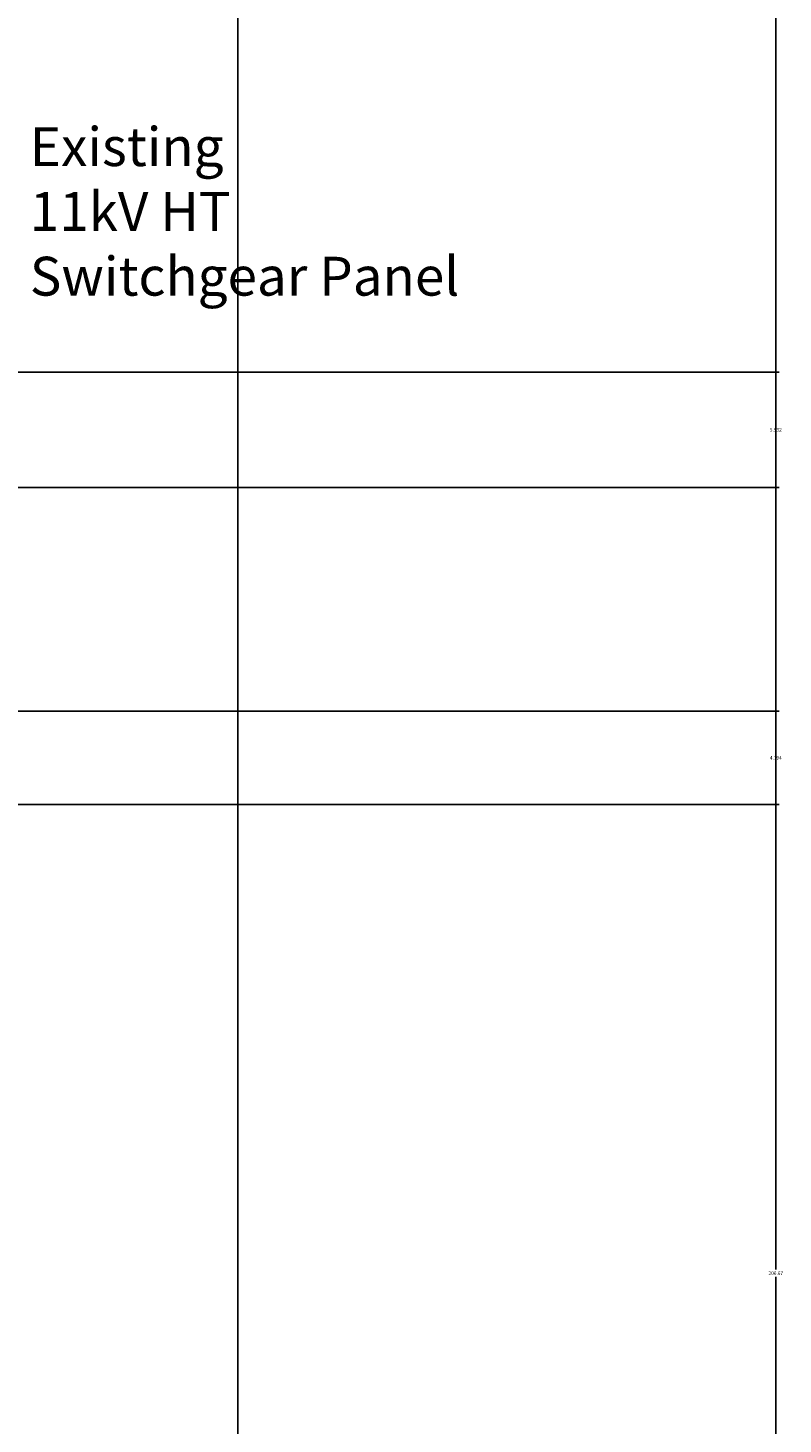
# Model space of a CAD drawing. Units: inches. Extents: x 412 to 584, y 208 to 437.
# Tile 22 of 28: x 545 to 584, y 315 to 387. Entities that reach past the tile are written whole.
import ezdxf

# ---------------------------------------------------------------- set-up
doc = ezdxf.new("R2010")
doc.units = ezdxf.units.IN
doc.header["$MEASUREMENT"] = 0
doc.layers.add('A-ANNO-DIMS', color=2, linetype='Continuous', lineweight=18)
doc.layers.add('E-ANNO-TEXT', color=7, linetype='Continuous', lineweight=18)
doc.styles.get("Standard").update_dxf_attribs({"font": 'arial.ttf'})
doc.dimstyles.get("Standard").update_dxf_attribs({"dimtxt": 0.18, "dimasz": 0.18, "dimexe": 0.18, "dimexo": 0.0625, "dimgap": 0.09, "dimtad": 0, "dimtih": 1, "dimtoh": 1, "dimdec": 4, "dimzin": 0, "dimdsep": 46, "dimtxsty": 'Standard', "dimcen": 0.09, "dimadec": 0, "dimazin": 0, "dimtfac": 1, "dimtdec": 4, "dimtofl": 0, "dimtmove": 0, "dimatfit": 3, "dimfxl": 1, "dimtolj": 1, "dimtzin": 0, "dimarcsym": 0})

# ---------------------------------------------------------------- blocks, each defined once
blk = doc.blocks.new('*D17')
at = {"layer": 'A-ANNO-DIMS', "color": 0, "lineweight": -2, "transparency": 16777216}
for p, q in [((497.715, 426.185), (583.674, 426.185)), ((583.494, 426.005), (583.494, 323.031)), ((583.494, 219.693), (583.494, 322.667)), ((550.198, 219.513), (583.674, 219.513))]:
    blk.add_line(p, q, dxfattribs=at)
at = {"layer": 'A-ANNO-DIMS', "color": 0, "transparency": 16777216}
for points in [[(583.464, 426.005), (583.524, 426.005), (583.494, 426.185)], [(583.464, 219.693), (583.524, 219.693), (583.494, 219.513)]]:
    blk.add_solid(points, dxfattribs=at)
at = {"layer": 'Defpoints', "color": 0, "transparency": 16777216}
for p in [(497.652, 426.185), (550.135, 219.513), (583.494, 219.513)]:
    blk.add_point(p, dxfattribs=at)
at = {"layer": 'A-ANNO-DIMS', "color": 0, "transparency": 16777216, "insert": (583.494, 322.849), "char_height": 0.18, "attachment_point": 5}
blk.add_mtext('\\A1;206.67', dxfattribs=at)
blk = doc.blocks.new('*D28')
at = {"layer": 'A-ANNO-DIMS', "color": 0, "lineweight": -2, "transparency": 16777216}
for p, q in [((450.562, 256.635), (450.562, 437.465)), ((450.742, 437.285), (502.724, 437.285)), ((555.616, 437.285), (503.634, 437.285)), ((555.796, 256.635), (555.796, 437.465))]:
    blk.add_line(p, q, dxfattribs=at)
at = {"layer": 'A-ANNO-DIMS', "color": 0, "transparency": 16777216}
for points in [[(450.742, 437.315), (450.742, 437.255), (450.562, 437.285)], [(555.616, 437.315), (555.616, 437.255), (555.796, 437.285)]]:
    blk.add_solid(points, dxfattribs=at)
at = {"layer": 'Defpoints', "color": 0, "transparency": 16777216}
for p in [(555.796, 437.285), (450.562, 256.573), (555.796, 256.573)]:
    blk.add_point(p, dxfattribs=at)
at = {"layer": 'A-ANNO-DIMS', "color": 0, "transparency": 16777216, "insert": (503.179, 437.285), "char_height": 0.18, "attachment_point": 5}
blk.add_mtext('\\A1;105.23', dxfattribs=at)
blk = doc.blocks.new('*D35')
at = {"layer": 'A-ANNO-DIMS', "color": 0, "lineweight": -2, "transparency": 16777216}
for p, q in [((485.523, 369.221), (583.674, 369.221)), ((583.494, 369.041), (583.494, 366.437)), ((583.494, 363.469), (583.494, 366.073)), ((485.523, 363.289), (583.674, 363.289))]:
    blk.add_line(p, q, dxfattribs=at)
at = {"layer": 'A-ANNO-DIMS', "color": 0, "transparency": 16777216}
for points in [[(583.464, 369.041), (583.524, 369.041), (583.494, 369.221)], [(583.464, 363.469), (583.524, 363.469), (583.494, 363.289)]]:
    blk.add_solid(points, dxfattribs=at)
at = {"layer": 'Defpoints', "color": 0, "transparency": 16777216}
for p in [(485.46, 369.221), (485.46, 363.289), (583.494, 363.289)]:
    blk.add_point(p, dxfattribs=at)
at = {"layer": 'A-ANNO-DIMS', "color": 0, "transparency": 16777216, "insert": (583.494, 366.255), "char_height": 0.18, "attachment_point": 5}
blk.add_mtext('\\A1;5.932', dxfattribs=at)
blk = doc.blocks.new('*D40')
at = {"layer": 'A-ANNO-DIMS', "color": 0, "lineweight": -2, "transparency": 16777216}
for p, q in [((501.747, 351.77), (583.674, 351.77)), ((583.494, 351.59), (583.494, 349.555)), ((583.494, 347.157), (583.494, 349.191)), ((501.747, 346.977), (583.674, 346.977))]:
    blk.add_line(p, q, dxfattribs=at)
at = {"layer": 'A-ANNO-DIMS', "color": 0, "transparency": 16777216}
for points in [[(583.464, 351.59), (583.524, 351.59), (583.494, 351.77)], [(583.464, 347.157), (583.524, 347.157), (583.494, 346.977)]]:
    blk.add_solid(points, dxfattribs=at)
at = {"layer": 'Defpoints', "color": 0, "transparency": 16777216}
for p in [(501.685, 351.77), (501.685, 346.977), (583.494, 346.977)]:
    blk.add_point(p, dxfattribs=at)
at = {"layer": 'A-ANNO-DIMS', "color": 0, "transparency": 16777216, "insert": (583.494, 349.373), "char_height": 0.18, "attachment_point": 5}
blk.add_mtext('\\A1;4.794', dxfattribs=at)

msp = doc.modelspace()

# ---------------------------------------------------------------- texts
at = {"layer": 'E-ANNO-TEXT', "insert": (545.0898, 381.8285), "char_height": 2, "attachment_point": 1}
msp.add_mtext_dynamic_manual_height_columns('\\pxql;Existing\\P11kV HT\\PSwitchgear Panel', width=26.749239, gutter_width=1, heights=[11.4418], dxfattribs=at)

# ---------------------------------------------------------------- dimensions: what is measured, and where the dimension line sits
at = {"layer": 'A-ANNO-DIMS'}
dim = msp.add_linear_dim(base=(555.7959, 437.2847), p1=(450.562, 256.5729), p2=(555.7959, 256.5729), dimstyle='Standard', override={"dimdec": 2, "dimlfac": 1, "dimrnd": 0, "dimzin": 0, "dimdsep": 46, "dimlunit": 2}, dxfattribs=at)
dim.commit()
dim.dimension.update_dxf_attribs({"geometry": '*D28', "text_midpoint": (503.1789, 437.2847)})
for base, p1, p2, override, picture, middle in [((583.4937, 219.5133), (497.6523, 426.1847), (550.1351, 219.5133), {"dimdec": 2, "dimlfac": 1, "dimrnd": 0, "dimzin": 0, "dimdsep": 46, "dimlunit": 2}, '*D17', (583.4937, 322.849)), ((583.4937, 363.2888), (485.4605, 369.221), (485.4605, 363.2888), {"dimdec": 3, "dimlfac": 1, "dimrnd": 0, "dimzin": 0, "dimdsep": 46, "dimlunit": 2}, '*D35', (583.4937, 366.2549)), ((583.4937, 346.9765), (501.6846, 351.7702), (501.6846, 346.9765), {"dimdec": 3, "dimlfac": 1, "dimrnd": 0, "dimzin": 0, "dimdsep": 46, "dimlunit": 2}, '*D40', (583.4937, 349.3734))]:
    dim = msp.add_linear_dim(base=base, p1=p1, p2=p2, angle=90, dimstyle='Standard', override=override, dxfattribs=at)
    dim.commit()
    dim.dimension.update_dxf_attribs({"geometry": picture, "text_midpoint": middle})

doc.saveas('drawing.dxf')
